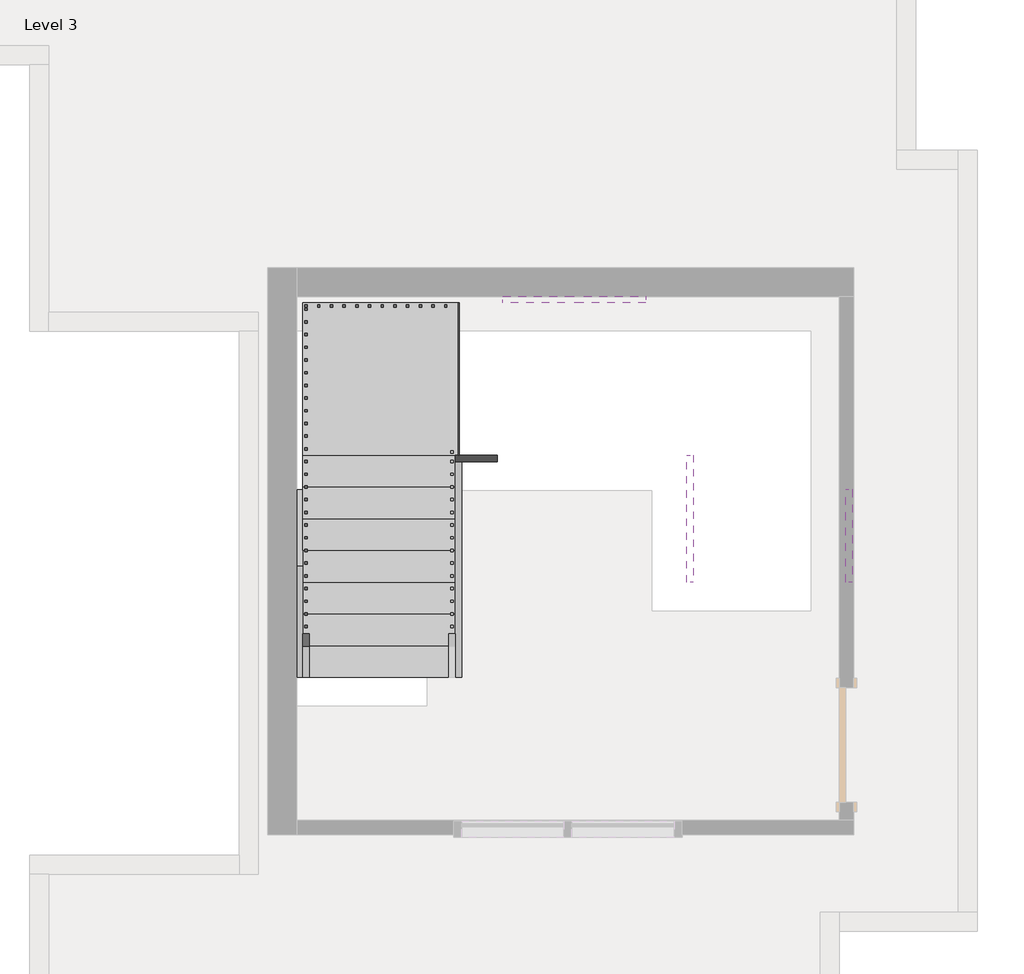
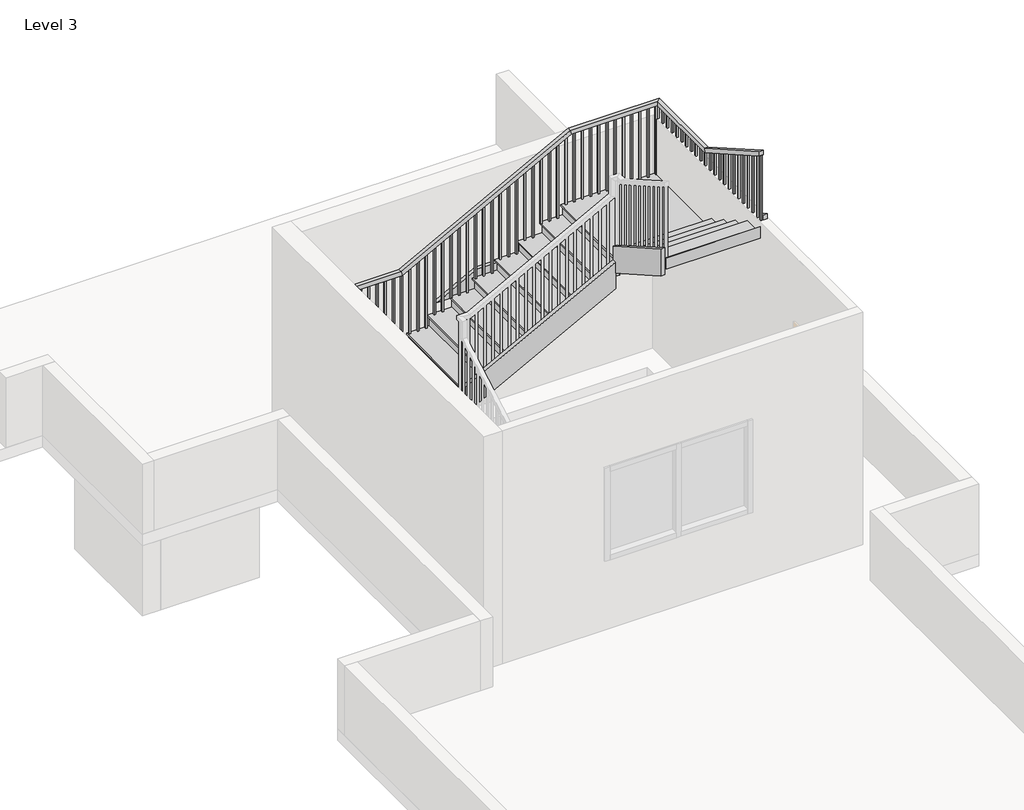
# One storey, part 2 of 2: 6 members, 1 railing, 1 stair flight.
"""IFC4 building model written with IfcOpenShell, lengths in millimetres."""

from ifc_helpers import new_model, si_unit, frame, origin, place, context, project, spatial, polyline, outline, extrude, faceted_brep, transform, mapped, element, save
from components import stair_flight_02d0fc9c

model = new_model("IFC4")

# Units and contexts
model_context = context("Model", 3, world=origin())
ifc_project = project(units=[si_unit("LENGTHUNIT", "METRE", prefix="MILLI")], contexts=[model_context])

# Site, building, storey
site = spatial("IfcSite", under=ifc_project)
building = spatial("IfcBuilding", under=site)
storey = spatial("IfcBuildingStorey", under=building, Name="Level 3", Elevation=6248.4)

# Members
placement = place(None, origin())
element("IfcMember", 1, ObjectType="Stringer - 2\" Width", at=placement, inside=storey, context=model_context, shape_type="SweptSolid", body=[
    extrude(outline(polyline([(12686.9618061, 6248.4), (12686.9618061, 6457.374685), (13575.3811074, 6965.0428571), (14189.7251478, 6965.0428571), (12935.6001478, 6248.4), (12686.9618061, 6248.4)])), frame((-40773.1146233, 0.0, 0.0), z_axis=(1.0, 0.0, 0.0), x_axis=(0.0, 1.0, 0.0)), (0.0, 0.0, 1.0), 50.8),
])
element("IfcMember", 2, ObjectType="Stringer - 2\" Width", at=placement, inside=storey, context=model_context, shape_type="SweptSolid", body=[
    extrude(outline(polyline([(7819.0066619, -38473.4324895), (8082.974685, -37978.4924462), (8082.974685, -38626.1924462), (7819.0066619, -39121.1324895), (7819.0066619, -38473.4324895)])), frame((0.0, 15684.1618061, 0.0), z_axis=(0.0, 1.0, 0.0), x_axis=(0.0, 0.0, 1.0)), (0.0, 0.0, 1.0), 50.8),
])
element("IfcMember", 3, ObjectType="Stringer - 2\" Width", at=placement, inside=storey, context=model_context, shape_type="SweptSolid", body=[
    extrude(outline(polyline([(13576.8784643, 8936.0828571), (13448.9618061, 9009.1780904), (13448.9618061, 9360.2318278), (14191.2225047, 8936.0828571), (13576.8784643, 8936.0828571)])), frame((-36378.9146233, 0.0, 0.0), z_axis=(1.0, 0.0, 0.0), x_axis=(0.0, 1.0, 0.0)), (0.0, 0.0, 1.0), 50.8),
])
element("IfcMember", 4, ObjectType="Stringer - 2\" Width", at=placement, inside=storey, context=model_context, shape_type="SweptSolid", body=[
    extrude(outline(polyline([(12686.9618061, 6248.4), (12686.9618061, 6457.374685), (14414.1618061, 7444.3461135), (14414.1618061, 7093.2923761), (12935.6001478, 6248.4), (12686.9618061, 6248.4)])), frame((-39503.1146233, 0.0, 0.0), z_axis=(1.0, 0.0, 0.0), x_axis=(0.0, 1.0, 0.0)), (0.0, 0.0, 1.0), 50.8),
])
element("IfcMember", 5, ObjectType="Stringer - 2\" Width", at=placement, inside=storey, context=model_context, shape_type="SweptSolid", body=[
    extrude(outline(polyline([(7615.2828571, -39503.1146233), (7269.8428571, -39503.1146233), (8258.7495238, -37648.9146233), (8604.1895238, -37648.9146233), (7615.2828571, -39503.1146233)])), frame((0.0, 14414.1618061, 0.0), z_axis=(0.0, 1.0, 0.0), x_axis=(0.0, 0.0, 1.0)), (0.0, 0.0, 1.0), 50.8),
])
element("IfcMember", 6, ObjectType="Stringer - 2\" Width", at=placement, inside=storey, context=model_context, shape_type="SweptSolid", body=[
    extrude(outline(polyline([(14464.9618061, 8779.6603992), (14464.9618061, 8428.6066619), (13448.9618061, 9009.1780904), (13448.9618061, 9360.2318278), (14464.9618061, 8779.6603992)])), frame((-37648.9146233, 0.0, 0.0), z_axis=(1.0, 0.0, 0.0), x_axis=(0.0, 1.0, 0.0)), (0.0, 0.0, 1.0), 50.8),
])

# Railing
element("IfcRailing", 7, ObjectType="Handrail - Rectangular", at=placement, inside=storey, context=model_context, shape_type="SolidModel", body=[
    faceted_brep([(-40722.3146233, 12686.9618061, 7307.9428571), (-40722.3146233, 12686.9618061, 7249.4339009), (-40671.5146233, 12686.9618061, 7249.4339009), (-40671.5146233, 12686.9618061, 7307.9428571), (-40722.3146233, 14631.7551394, 8419.2533333), (-40722.3146233, 14645.2458128, 8368.4533333), (-40671.5146233, 14645.2458128, 8368.4533333), (-40671.5146233, 14631.7551394, 8419.2533333), (-40722.3146233, 15684.1618061, 8419.2533333), (-40722.3146233, 15684.1618061, 8368.4533333), (-40671.5146233, 15633.3618061, 8368.4533333), (-40671.5146233, 15633.3618061, 8419.2533333), (-39596.5503376, 15684.1618061, 8419.2533333), (-39583.8503376, 15684.1618061, 8368.4533333), (-39583.8503376, 15633.3618061, 8368.4533333), (-39596.5503376, 15633.3618061, 8419.2533333), (-37504.6789091, 15684.1618061, 9534.9180952), (-37491.9789091, 15684.1618061, 9484.1180952), (-37491.9789091, 15633.3618061, 9484.1180952), (-37504.6789091, 15633.3618061, 9534.9180952), (-36378.9146233, 15684.1618061, 9534.9180952), (-36378.9146233, 15684.1618061, 9484.1180952), (-36429.7146233, 15633.3618061, 9484.1180952), (-36429.7146233, 15633.3618061, 9534.9180952), (-36378.9146233, 14631.7551394, 9534.9180952), (-36378.9146233, 14618.264466, 9484.1180952), (-36429.7146233, 14618.264466, 9484.1180952), (-36429.7146233, 14631.7551394, 9534.9180952), (-36378.9146233, 13448.9618061, 10210.8), (-36429.7146233, 13448.9618061, 10210.8), (-36429.7146233, 13448.9618061, 10152.2910438), (-36378.9146233, 13448.9618061, 10152.2910438)], [[[0, 1, 2, 3]], [[1, 0, 4, 5]], [[2, 1, 5, 6]], [[3, 2, 6, 7]], [[0, 3, 7, 4]], [[5, 4, 8, 9]], [[6, 5, 9, 10]], [[7, 6, 10, 11]], [[4, 7, 11, 8]], [[9, 8, 12, 13]], [[10, 9, 13, 14]], [[11, 10, 14, 15]], [[8, 11, 15, 12]], [[13, 12, 16, 17]], [[14, 13, 17, 18]], [[15, 14, 18, 19]], [[12, 15, 19, 16]], [[17, 16, 20, 21]], [[18, 17, 21, 22]], [[19, 18, 22, 23]], [[16, 19, 23, 20]], [[21, 20, 24, 25]], [[22, 21, 25, 26]], [[23, 22, 26, 27]], [[20, 23, 27, 24]], [[28, 29, 30, 31]], [[25, 24, 28, 31]], [[26, 25, 31, 30]], [[27, 26, 30, 29]], [[24, 27, 29, 28]]]),
    extrude(outline(polyline([(13534.6868061, 10103.3053295), (13534.6868061, 9151.2571429), (13515.6368061, 9151.2571429), (13515.6368061, 10114.1910438), (13534.6868061, 10103.3053295)])), frame((-36413.8396233, 0.0, 0.0), z_axis=(1.0, 0.0, 0.0), x_axis=(0.0, 1.0, 0.0)), (0.0, 0.0, 1.0), 19.05),
    extrude(outline(polyline([(13636.2868061, 10045.2481866), (13636.2868061, 9151.2571429), (13617.2368061, 9151.2571429), (13617.2368061, 10056.1339009), (13636.2868061, 10045.2481866)])), frame((-36413.8396233, 0.0, 0.0), z_axis=(1.0, 0.0, 0.0), x_axis=(0.0, 1.0, 0.0)), (0.0, 0.0, 1.0), 19.05),
    extrude(outline(polyline([(13737.8868061, 9987.1910438), (13737.8868061, 9006.1142857), (13718.8368061, 9006.1142857), (13718.8368061, 9998.0767581), (13737.8868061, 9987.1910438)])), frame((-36413.8396233, 0.0, 0.0), z_axis=(1.0, 0.0, 0.0), x_axis=(0.0, 1.0, 0.0)), (0.0, 0.0, 1.0), 19.05),
    extrude(outline(polyline([(13839.4868061, 9929.1339009), (13839.4868061, 9006.1142857), (13820.4368061, 9006.1142857), (13820.4368061, 9940.0196152), (13839.4868061, 9929.1339009)])), frame((-36413.8396233, 0.0, 0.0), z_axis=(1.0, 0.0, 0.0), x_axis=(0.0, 1.0, 0.0)), (0.0, 0.0, 1.0), 19.05),
    extrude(outline(polyline([(13941.0868061, 9871.0767581), (13941.0868061, 9006.1142857), (13922.0368061, 9006.1142857), (13922.0368061, 9881.9624723), (13941.0868061, 9871.0767581)])), frame((-36413.8396233, 0.0, 0.0), z_axis=(1.0, 0.0, 0.0), x_axis=(0.0, 1.0, 0.0)), (0.0, 0.0, 1.0), 19.05),
    extrude(outline(polyline([(14042.6868061, 9813.0196152), (14042.6868061, 8860.9714286), (14023.6368061, 8860.9714286), (14023.6368061, 9823.9053295), (14042.6868061, 9813.0196152)])), frame((-36413.8396233, 0.0, 0.0), z_axis=(1.0, 0.0, 0.0), x_axis=(0.0, 1.0, 0.0)), (0.0, 0.0, 1.0), 19.05),
    extrude(outline(polyline([(14144.2868061, 9754.9624723), (14144.2868061, 8860.9714286), (14125.2368061, 8860.9714286), (14125.2368061, 9765.8481866), (14144.2868061, 9754.9624723)])), frame((-36413.8396233, 0.0, 0.0), z_axis=(1.0, 0.0, 0.0), x_axis=(0.0, 1.0, 0.0)), (0.0, 0.0, 1.0), 19.05),
    extrude(outline(polyline([(14245.8868061, 9696.9053295), (14245.8868061, 8715.8285714), (14226.8368061, 8715.8285714), (14226.8368061, 9707.7910438), (14245.8868061, 9696.9053295)])), frame((-36413.8396233, 0.0, 0.0), z_axis=(1.0, 0.0, 0.0), x_axis=(0.0, 1.0, 0.0)), (0.0, 0.0, 1.0), 19.05),
    extrude(outline(polyline([(14347.4868061, 9638.8481866), (14347.4868061, 8715.8285714), (14328.4368061, 8715.8285714), (14328.4368061, 9649.7339009), (14347.4868061, 9638.8481866)])), frame((-36413.8396233, 0.0, 0.0), z_axis=(1.0, 0.0, 0.0), x_axis=(0.0, 1.0, 0.0)), (0.0, 0.0, 1.0), 19.05),
    extrude(outline(polyline([(14449.0868061, 9580.7910438), (14449.0868061, 8715.8285714), (14430.0368061, 8715.8285714), (14430.0368061, 9591.6767581), (14449.0868061, 9580.7910438)])), frame((-36413.8396233, 0.0, 0.0), z_axis=(1.0, 0.0, 0.0), x_axis=(0.0, 1.0, 0.0)), (0.0, 0.0, 1.0), 19.05),
    extrude(outline(polyline([(14550.6868061, 9522.7339009), (14550.6868061, 8570.6857143), (14531.6368061, 8570.6857143), (14531.6368061, 9533.6196152), (14550.6868061, 9522.7339009)])), frame((-36413.8396233, 0.0, 0.0), z_axis=(1.0, 0.0, 0.0), x_axis=(0.0, 1.0, 0.0)), (0.0, 0.0, 1.0), 19.05),
    extrude(outline(polyline([(-36394.7896233, 14652.2868061), (-36394.7896233, 14633.2368061), (-36413.8396233, 14633.2368061), (-36413.8396233, 14652.2868061), (-36394.7896233, 14652.2868061)])), frame((0.0, 0.0, 8570.6857143), z_axis=(0.0, 0.0, 1.0), x_axis=(1.0, 0.0, 0.0)), (0.0, 0.0, 1.0), 913.432381),
    extrude(outline(polyline([(-36394.7896233, 14753.8868061), (-36394.7896233, 14734.8368061), (-36413.8396233, 14734.8368061), (-36413.8396233, 14753.8868061), (-36394.7896233, 14753.8868061)])), frame((0.0, 0.0, 8570.6857143), z_axis=(0.0, 0.0, 1.0), x_axis=(1.0, 0.0, 0.0)), (0.0, 0.0, 1.0), 913.432381),
    extrude(outline(polyline([(-36394.7896233, 14855.4868061), (-36394.7896233, 14836.4368061), (-36413.8396233, 14836.4368061), (-36413.8396233, 14855.4868061), (-36394.7896233, 14855.4868061)])), frame((0.0, 0.0, 8570.6857143), z_axis=(0.0, 0.0, 1.0), x_axis=(1.0, 0.0, 0.0)), (0.0, 0.0, 1.0), 913.432381),
    extrude(outline(polyline([(-36394.7896233, 14957.0868061), (-36394.7896233, 14938.0368061), (-36413.8396233, 14938.0368061), (-36413.8396233, 14957.0868061), (-36394.7896233, 14957.0868061)])), frame((0.0, 0.0, 8570.6857143), z_axis=(0.0, 0.0, 1.0), x_axis=(1.0, 0.0, 0.0)), (0.0, 0.0, 1.0), 913.432381),
    extrude(outline(polyline([(-36394.7896233, 15058.6868061), (-36394.7896233, 15039.6368061), (-36413.8396233, 15039.6368061), (-36413.8396233, 15058.6868061), (-36394.7896233, 15058.6868061)])), frame((0.0, 0.0, 8570.6857143), z_axis=(0.0, 0.0, 1.0), x_axis=(1.0, 0.0, 0.0)), (0.0, 0.0, 1.0), 913.432381),
    extrude(outline(polyline([(-36394.7896233, 15160.2868061), (-36394.7896233, 15141.2368061), (-36413.8396233, 15141.2368061), (-36413.8396233, 15160.2868061), (-36394.7896233, 15160.2868061)])), frame((0.0, 0.0, 8570.6857143), z_axis=(0.0, 0.0, 1.0), x_axis=(1.0, 0.0, 0.0)), (0.0, 0.0, 1.0), 913.432381),
    extrude(outline(polyline([(-36394.7896233, 15261.8868061), (-36394.7896233, 15242.8368061), (-36413.8396233, 15242.8368061), (-36413.8396233, 15261.8868061), (-36394.7896233, 15261.8868061)])), frame((0.0, 0.0, 8570.6857143), z_axis=(0.0, 0.0, 1.0), x_axis=(1.0, 0.0, 0.0)), (0.0, 0.0, 1.0), 913.432381),
    extrude(outline(polyline([(-36394.7896233, 15363.4868061), (-36394.7896233, 15344.4368061), (-36413.8396233, 15344.4368061), (-36413.8396233, 15363.4868061), (-36394.7896233, 15363.4868061)])), frame((0.0, 0.0, 8570.6857143), z_axis=(0.0, 0.0, 1.0), x_axis=(1.0, 0.0, 0.0)), (0.0, 0.0, 1.0), 913.432381),
    extrude(outline(polyline([(-36394.7896233, 15465.0868061), (-36394.7896233, 15446.0368061), (-36413.8396233, 15446.0368061), (-36413.8396233, 15465.0868061), (-36394.7896233, 15465.0868061)])), frame((0.0, 0.0, 8570.6857143), z_axis=(0.0, 0.0, 1.0), x_axis=(1.0, 0.0, 0.0)), (0.0, 0.0, 1.0), 913.432381),
    extrude(outline(polyline([(-36394.7896233, 15566.6868061), (-36394.7896233, 15547.6368061), (-36413.8396233, 15547.6368061), (-36413.8396233, 15566.6868061), (-36394.7896233, 15566.6868061)])), frame((0.0, 0.0, 8570.6857143), z_axis=(0.0, 0.0, 1.0), x_axis=(1.0, 0.0, 0.0)), (0.0, 0.0, 1.0), 913.432381),
    extrude(outline(polyline([(-36439.2396233, 15668.2868061), (-36420.1896233, 15668.2868061), (-36420.1896233, 15649.2368061), (-36439.2396233, 15649.2368061), (-36439.2396233, 15668.2868061)])), frame((0.0, 0.0, 8570.6857143), z_axis=(0.0, 0.0, 1.0), x_axis=(1.0, 0.0, 0.0)), (0.0, 0.0, 1.0), 913.432381),
    extrude(outline(polyline([(-36540.8396233, 15668.2868061), (-36521.7896233, 15668.2868061), (-36521.7896233, 15649.2368061), (-36540.8396233, 15649.2368061), (-36540.8396233, 15668.2868061)])), frame((0.0, 0.0, 8570.6857143), z_axis=(0.0, 0.0, 1.0), x_axis=(1.0, 0.0, 0.0)), (0.0, 0.0, 1.0), 913.432381),
    extrude(outline(polyline([(-36642.4396233, 15668.2868061), (-36623.3896233, 15668.2868061), (-36623.3896233, 15649.2368061), (-36642.4396233, 15649.2368061), (-36642.4396233, 15668.2868061)])), frame((0.0, 0.0, 8570.6857143), z_axis=(0.0, 0.0, 1.0), x_axis=(1.0, 0.0, 0.0)), (0.0, 0.0, 1.0), 913.432381),
    extrude(outline(polyline([(-36744.0396233, 15668.2868061), (-36724.9896233, 15668.2868061), (-36724.9896233, 15649.2368061), (-36744.0396233, 15649.2368061), (-36744.0396233, 15668.2868061)])), frame((0.0, 0.0, 8570.6857143), z_axis=(0.0, 0.0, 1.0), x_axis=(1.0, 0.0, 0.0)), (0.0, 0.0, 1.0), 913.432381),
    extrude(outline(polyline([(-36845.6396233, 15668.2868061), (-36826.5896233, 15668.2868061), (-36826.5896233, 15649.2368061), (-36845.6396233, 15649.2368061), (-36845.6396233, 15668.2868061)])), frame((0.0, 0.0, 8570.6857143), z_axis=(0.0, 0.0, 1.0), x_axis=(1.0, 0.0, 0.0)), (0.0, 0.0, 1.0), 913.432381),
    extrude(outline(polyline([(-36947.2396233, 15668.2868061), (-36928.1896233, 15668.2868061), (-36928.1896233, 15649.2368061), (-36947.2396233, 15649.2368061), (-36947.2396233, 15668.2868061)])), frame((0.0, 0.0, 8570.6857143), z_axis=(0.0, 0.0, 1.0), x_axis=(1.0, 0.0, 0.0)), (0.0, 0.0, 1.0), 913.432381),
    extrude(outline(polyline([(-37048.8396233, 15668.2868061), (-37029.7896233, 15668.2868061), (-37029.7896233, 15649.2368061), (-37048.8396233, 15649.2368061), (-37048.8396233, 15668.2868061)])), frame((0.0, 0.0, 8570.6857143), z_axis=(0.0, 0.0, 1.0), x_axis=(1.0, 0.0, 0.0)), (0.0, 0.0, 1.0), 913.432381),
    extrude(outline(polyline([(-37150.4396233, 15668.2868061), (-37131.3896233, 15668.2868061), (-37131.3896233, 15649.2368061), (-37150.4396233, 15649.2368061), (-37150.4396233, 15668.2868061)])), frame((0.0, 0.0, 8570.6857143), z_axis=(0.0, 0.0, 1.0), x_axis=(1.0, 0.0, 0.0)), (0.0, 0.0, 1.0), 913.432381),
    extrude(outline(polyline([(-37252.0396233, 15668.2868061), (-37232.9896233, 15668.2868061), (-37232.9896233, 15649.2368061), (-37252.0396233, 15649.2368061), (-37252.0396233, 15668.2868061)])), frame((0.0, 0.0, 8570.6857143), z_axis=(0.0, 0.0, 1.0), x_axis=(1.0, 0.0, 0.0)), (0.0, 0.0, 1.0), 913.432381),
    extrude(outline(polyline([(-37353.6396233, 15668.2868061), (-37334.5896233, 15668.2868061), (-37334.5896233, 15649.2368061), (-37353.6396233, 15649.2368061), (-37353.6396233, 15668.2868061)])), frame((0.0, 0.0, 8570.6857143), z_axis=(0.0, 0.0, 1.0), x_axis=(1.0, 0.0, 0.0)), (0.0, 0.0, 1.0), 913.432381),
    extrude(outline(polyline([(-37455.2396233, 15668.2868061), (-37436.1896233, 15668.2868061), (-37436.1896233, 15649.2368061), (-37455.2396233, 15649.2368061), (-37455.2396233, 15668.2868061)])), frame((0.0, 0.0, 8570.6857143), z_axis=(0.0, 0.0, 1.0), x_axis=(1.0, 0.0, 0.0)), (0.0, 0.0, 1.0), 913.432381),
    extrude(outline(polyline([(9449.5257143, -37556.8396233), (8570.6857143, -37556.8396233), (8570.6857143, -37537.7896233), (9459.6857143, -37537.7896233), (9449.5257143, -37556.8396233)])), frame((0.0, 15649.2368061, 0.0), z_axis=(0.0, 1.0, 0.0), x_axis=(0.0, 0.0, 1.0)), (0.0, 0.0, 1.0), 19.05),
    extrude(outline(polyline([(9395.3390476, -37658.4396233), (8425.5428571, -37658.4396233), (8425.5428571, -37639.3896233), (9405.4990476, -37639.3896233), (9395.3390476, -37658.4396233)])), frame((0.0, 15649.2368061, 0.0), z_axis=(0.0, 1.0, 0.0), x_axis=(0.0, 0.0, 1.0)), (0.0, 0.0, 1.0), 19.05),
    extrude(outline(polyline([(9341.152381, -37760.0396233), (8425.5428571, -37760.0396233), (8425.5428571, -37740.9896233), (9351.312381, -37740.9896233), (9341.152381, -37760.0396233)])), frame((0.0, 15649.2368061, 0.0), z_axis=(0.0, 1.0, 0.0), x_axis=(0.0, 0.0, 1.0)), (0.0, 0.0, 1.0), 19.05),
    extrude(outline(polyline([(9286.9657143, -37861.6396233), (8425.5428571, -37861.6396233), (8425.5428571, -37842.5896233), (9297.1257143, -37842.5896233), (9286.9657143, -37861.6396233)])), frame((0.0, 15649.2368061, 0.0), z_axis=(0.0, 1.0, 0.0), x_axis=(0.0, 0.0, 1.0)), (0.0, 0.0, 1.0), 19.05),
    extrude(outline(polyline([(9232.7790476, -37963.2396233), (8280.4, -37963.2396233), (8280.4, -37944.1896233), (9242.9390476, -37944.1896233), (9232.7790476, -37963.2396233)])), frame((0.0, 15649.2368061, 0.0), z_axis=(0.0, 1.0, 0.0), x_axis=(0.0, 0.0, 1.0)), (0.0, 0.0, 1.0), 19.05),
    extrude(outline(polyline([(9178.592381, -38064.8396233), (8280.4, -38064.8396233), (8280.4, -38045.7896233), (9188.752381, -38045.7896233), (9178.592381, -38064.8396233)])), frame((0.0, 15649.2368061, 0.0), z_axis=(0.0, 1.0, 0.0), x_axis=(0.0, 0.0, 1.0)), (0.0, 0.0, 1.0), 19.05),
    extrude(outline(polyline([(9124.4057143, -38166.4396233), (8135.2571429, -38166.4396233), (8135.2571429, -38147.3896233), (9134.5657143, -38147.3896233), (9124.4057143, -38166.4396233)])), frame((0.0, 15649.2368061, 0.0), z_axis=(0.0, 1.0, 0.0), x_axis=(0.0, 0.0, 1.0)), (0.0, 0.0, 1.0), 19.05),
    extrude(outline(polyline([(9070.2190476, -38268.0396233), (8135.2571429, -38268.0396233), (8135.2571429, -38248.9896233), (9080.3790476, -38248.9896233), (9070.2190476, -38268.0396233)])), frame((0.0, 15649.2368061, 0.0), z_axis=(0.0, 1.0, 0.0), x_axis=(0.0, 0.0, 1.0)), (0.0, 0.0, 1.0), 19.05),
    extrude(outline(polyline([(9016.032381, -38369.6396233), (8135.2571429, -38369.6396233), (8135.2571429, -38350.5896233), (9026.192381, -38350.5896233), (9016.032381, -38369.6396233)])), frame((0.0, 15649.2368061, 0.0), z_axis=(0.0, 1.0, 0.0), x_axis=(0.0, 0.0, 1.0)), (0.0, 0.0, 1.0), 19.05),
    extrude(outline(polyline([(8961.8457143, -38471.2396233), (7990.1142857, -38471.2396233), (7990.1142857, -38452.1896233), (8972.0057143, -38452.1896233), (8961.8457143, -38471.2396233)])), frame((0.0, 15649.2368061, 0.0), z_axis=(0.0, 1.0, 0.0), x_axis=(0.0, 0.0, 1.0)), (0.0, 0.0, 1.0), 19.05),
    extrude(outline(polyline([(8907.6590476, -38572.8396233), (7990.1142857, -38572.8396233), (7990.1142857, -38553.7896233), (8917.8190476, -38553.7896233), (8907.6590476, -38572.8396233)])), frame((0.0, 15649.2368061, 0.0), z_axis=(0.0, 1.0, 0.0), x_axis=(0.0, 0.0, 1.0)), (0.0, 0.0, 1.0), 19.05),
    extrude(outline(polyline([(8853.472381, -38674.4396233), (7990.1142857, -38674.4396233), (7990.1142857, -38655.3896233), (8863.632381, -38655.3896233), (8853.472381, -38674.4396233)])), frame((0.0, 15649.2368061, 0.0), z_axis=(0.0, 1.0, 0.0), x_axis=(0.0, 0.0, 1.0)), (0.0, 0.0, 1.0), 19.05),
    extrude(outline(polyline([(8799.2857143, -38776.0396233), (7844.9714286, -38776.0396233), (7844.9714286, -38756.9896233), (8809.4457143, -38756.9896233), (8799.2857143, -38776.0396233)])), frame((0.0, 15649.2368061, 0.0), z_axis=(0.0, 1.0, 0.0), x_axis=(0.0, 0.0, 1.0)), (0.0, 0.0, 1.0), 19.05),
    extrude(outline(polyline([(8745.0990476, -38877.6396233), (7844.9714286, -38877.6396233), (7844.9714286, -38858.5896233), (8755.2590476, -38858.5896233), (8745.0990476, -38877.6396233)])), frame((0.0, 15649.2368061, 0.0), z_axis=(0.0, 1.0, 0.0), x_axis=(0.0, 0.0, 1.0)), (0.0, 0.0, 1.0), 19.05),
    extrude(outline(polyline([(8690.912381, -38979.2396233), (7844.9714286, -38979.2396233), (7844.9714286, -38960.1896233), (8701.072381, -38960.1896233), (8690.912381, -38979.2396233)])), frame((0.0, 15649.2368061, 0.0), z_axis=(0.0, 1.0, 0.0), x_axis=(0.0, 0.0, 1.0)), (0.0, 0.0, 1.0), 19.05),
    extrude(outline(polyline([(8636.7257143, -39080.8396233), (7699.8285714, -39080.8396233), (7699.8285714, -39061.7896233), (8646.8857143, -39061.7896233), (8636.7257143, -39080.8396233)])), frame((0.0, 15649.2368061, 0.0), z_axis=(0.0, 1.0, 0.0), x_axis=(0.0, 0.0, 1.0)), (0.0, 0.0, 1.0), 19.05),
    extrude(outline(polyline([(8582.5390476, -39182.4396233), (7699.8285714, -39182.4396233), (7699.8285714, -39163.3896233), (8592.6990476, -39163.3896233), (8582.5390476, -39182.4396233)])), frame((0.0, 15649.2368061, 0.0), z_axis=(0.0, 1.0, 0.0), x_axis=(0.0, 0.0, 1.0)), (0.0, 0.0, 1.0), 19.05),
    extrude(outline(polyline([(8528.352381, -39284.0396233), (7554.6857143, -39284.0396233), (7554.6857143, -39264.9896233), (8538.512381, -39264.9896233), (8528.352381, -39284.0396233)])), frame((0.0, 15649.2368061, 0.0), z_axis=(0.0, 1.0, 0.0), x_axis=(0.0, 0.0, 1.0)), (0.0, 0.0, 1.0), 19.05),
    extrude(outline(polyline([(8474.1657143, -39385.6396233), (7554.6857143, -39385.6396233), (7554.6857143, -39366.5896233), (8484.3257143, -39366.5896233), (8474.1657143, -39385.6396233)])), frame((0.0, 15649.2368061, 0.0), z_axis=(0.0, 1.0, 0.0), x_axis=(0.0, 0.0, 1.0)), (0.0, 0.0, 1.0), 19.05),
    extrude(outline(polyline([(8419.9790476, -39487.2396233), (7554.6857143, -39487.2396233), (7554.6857143, -39468.1896233), (8430.1390476, -39468.1896233), (8419.9790476, -39487.2396233)])), frame((0.0, 15649.2368061, 0.0), z_axis=(0.0, 1.0, 0.0), x_axis=(0.0, 0.0, 1.0)), (0.0, 0.0, 1.0), 19.05),
    extrude(outline(polyline([(8365.792381, -39588.8396233), (7409.5428571, -39588.8396233), (7409.5428571, -39569.7896233), (8375.952381, -39569.7896233), (8365.792381, -39588.8396233)])), frame((0.0, 15649.2368061, 0.0), z_axis=(0.0, 1.0, 0.0), x_axis=(0.0, 0.0, 1.0)), (0.0, 0.0, 1.0), 19.05),
    extrude(outline(polyline([(-39690.4396233, 15668.2868061), (-39671.3896233, 15668.2868061), (-39671.3896233, 15649.2368061), (-39690.4396233, 15649.2368061), (-39690.4396233, 15668.2868061)])), frame((0.0, 0.0, 7409.5428571), z_axis=(0.0, 0.0, 1.0), x_axis=(1.0, 0.0, 0.0)), (0.0, 0.0, 1.0), 958.9104762),
    extrude(outline(polyline([(-39792.0396233, 15668.2868061), (-39772.9896233, 15668.2868061), (-39772.9896233, 15649.2368061), (-39792.0396233, 15649.2368061), (-39792.0396233, 15668.2868061)])), frame((0.0, 0.0, 7409.5428571), z_axis=(0.0, 0.0, 1.0), x_axis=(1.0, 0.0, 0.0)), (0.0, 0.0, 1.0), 958.9104762),
    extrude(outline(polyline([(-39893.6396233, 15668.2868061), (-39874.5896233, 15668.2868061), (-39874.5896233, 15649.2368061), (-39893.6396233, 15649.2368061), (-39893.6396233, 15668.2868061)])), frame((0.0, 0.0, 7409.5428571), z_axis=(0.0, 0.0, 1.0), x_axis=(1.0, 0.0, 0.0)), (0.0, 0.0, 1.0), 958.9104762),
    extrude(outline(polyline([(-39995.2396233, 15668.2868061), (-39976.1896233, 15668.2868061), (-39976.1896233, 15649.2368061), (-39995.2396233, 15649.2368061), (-39995.2396233, 15668.2868061)])), frame((0.0, 0.0, 7409.5428571), z_axis=(0.0, 0.0, 1.0), x_axis=(1.0, 0.0, 0.0)), (0.0, 0.0, 1.0), 958.9104762),
    extrude(outline(polyline([(-40096.8396233, 15668.2868061), (-40077.7896233, 15668.2868061), (-40077.7896233, 15649.2368061), (-40096.8396233, 15649.2368061), (-40096.8396233, 15668.2868061)])), frame((0.0, 0.0, 7409.5428571), z_axis=(0.0, 0.0, 1.0), x_axis=(1.0, 0.0, 0.0)), (0.0, 0.0, 1.0), 958.9104762),
    extrude(outline(polyline([(-40198.4396233, 15668.2868061), (-40179.3896233, 15668.2868061), (-40179.3896233, 15649.2368061), (-40198.4396233, 15649.2368061), (-40198.4396233, 15668.2868061)])), frame((0.0, 0.0, 7409.5428571), z_axis=(0.0, 0.0, 1.0), x_axis=(1.0, 0.0, 0.0)), (0.0, 0.0, 1.0), 958.9104762),
    extrude(outline(polyline([(-40300.0396233, 15668.2868061), (-40280.9896233, 15668.2868061), (-40280.9896233, 15649.2368061), (-40300.0396233, 15649.2368061), (-40300.0396233, 15668.2868061)])), frame((0.0, 0.0, 7409.5428571), z_axis=(0.0, 0.0, 1.0), x_axis=(1.0, 0.0, 0.0)), (0.0, 0.0, 1.0), 958.9104762),
    extrude(outline(polyline([(-40401.6396233, 15668.2868061), (-40382.5896233, 15668.2868061), (-40382.5896233, 15649.2368061), (-40401.6396233, 15649.2368061), (-40401.6396233, 15668.2868061)])), frame((0.0, 0.0, 7409.5428571), z_axis=(0.0, 0.0, 1.0), x_axis=(1.0, 0.0, 0.0)), (0.0, 0.0, 1.0), 958.9104762),
    extrude(outline(polyline([(-40503.2396233, 15668.2868061), (-40484.1896233, 15668.2868061), (-40484.1896233, 15649.2368061), (-40503.2396233, 15649.2368061), (-40503.2396233, 15668.2868061)])), frame((0.0, 0.0, 7409.5428571), z_axis=(0.0, 0.0, 1.0), x_axis=(1.0, 0.0, 0.0)), (0.0, 0.0, 1.0), 958.9104762),
    extrude(outline(polyline([(-40604.8396233, 15668.2868061), (-40585.7896233, 15668.2868061), (-40585.7896233, 15649.2368061), (-40604.8396233, 15649.2368061), (-40604.8396233, 15668.2868061)])), frame((0.0, 0.0, 7409.5428571), z_axis=(0.0, 0.0, 1.0), x_axis=(1.0, 0.0, 0.0)), (0.0, 0.0, 1.0), 958.9104762),
    extrude(outline(polyline([(-40706.4396233, 15623.8368061), (-40706.4396233, 15642.8868061), (-40687.3896233, 15642.8868061), (-40687.3896233, 15623.8368061), (-40706.4396233, 15623.8368061)])), frame((0.0, 0.0, 7409.5428571), z_axis=(0.0, 0.0, 1.0), x_axis=(1.0, 0.0, 0.0)), (0.0, 0.0, 1.0), 958.9104762),
    extrude(outline(polyline([(-40706.4396233, 15522.2368061), (-40706.4396233, 15541.2868061), (-40687.3896233, 15541.2868061), (-40687.3896233, 15522.2368061), (-40706.4396233, 15522.2368061)])), frame((0.0, 0.0, 7409.5428571), z_axis=(0.0, 0.0, 1.0), x_axis=(1.0, 0.0, 0.0)), (0.0, 0.0, 1.0), 958.9104762),
    extrude(outline(polyline([(-40706.4396233, 15420.6368061), (-40706.4396233, 15439.6868061), (-40687.3896233, 15439.6868061), (-40687.3896233, 15420.6368061), (-40706.4396233, 15420.6368061)])), frame((0.0, 0.0, 7409.5428571), z_axis=(0.0, 0.0, 1.0), x_axis=(1.0, 0.0, 0.0)), (0.0, 0.0, 1.0), 958.9104762),
    extrude(outline(polyline([(-40706.4396233, 15319.0368061), (-40706.4396233, 15338.0868061), (-40687.3896233, 15338.0868061), (-40687.3896233, 15319.0368061), (-40706.4396233, 15319.0368061)])), frame((0.0, 0.0, 7409.5428571), z_axis=(0.0, 0.0, 1.0), x_axis=(1.0, 0.0, 0.0)), (0.0, 0.0, 1.0), 958.9104762),
    extrude(outline(polyline([(-40706.4396233, 15217.4368061), (-40706.4396233, 15236.4868061), (-40687.3896233, 15236.4868061), (-40687.3896233, 15217.4368061), (-40706.4396233, 15217.4368061)])), frame((0.0, 0.0, 7409.5428571), z_axis=(0.0, 0.0, 1.0), x_axis=(1.0, 0.0, 0.0)), (0.0, 0.0, 1.0), 958.9104762),
    extrude(outline(polyline([(-40706.4396233, 15115.8368061), (-40706.4396233, 15134.8868061), (-40687.3896233, 15134.8868061), (-40687.3896233, 15115.8368061), (-40706.4396233, 15115.8368061)])), frame((0.0, 0.0, 7409.5428571), z_axis=(0.0, 0.0, 1.0), x_axis=(1.0, 0.0, 0.0)), (0.0, 0.0, 1.0), 958.9104762),
    extrude(outline(polyline([(-40706.4396233, 15014.2368061), (-40706.4396233, 15033.2868061), (-40687.3896233, 15033.2868061), (-40687.3896233, 15014.2368061), (-40706.4396233, 15014.2368061)])), frame((0.0, 0.0, 7409.5428571), z_axis=(0.0, 0.0, 1.0), x_axis=(1.0, 0.0, 0.0)), (0.0, 0.0, 1.0), 958.9104762),
    extrude(outline(polyline([(-40706.4396233, 14912.6368061), (-40706.4396233, 14931.6868061), (-40687.3896233, 14931.6868061), (-40687.3896233, 14912.6368061), (-40706.4396233, 14912.6368061)])), frame((0.0, 0.0, 7409.5428571), z_axis=(0.0, 0.0, 1.0), x_axis=(1.0, 0.0, 0.0)), (0.0, 0.0, 1.0), 958.9104762),
    extrude(outline(polyline([(-40706.4396233, 14811.0368061), (-40706.4396233, 14830.0868061), (-40687.3896233, 14830.0868061), (-40687.3896233, 14811.0368061), (-40706.4396233, 14811.0368061)])), frame((0.0, 0.0, 7409.5428571), z_axis=(0.0, 0.0, 1.0), x_axis=(1.0, 0.0, 0.0)), (0.0, 0.0, 1.0), 958.9104762),
    extrude(outline(polyline([(-40706.4396233, 14709.4368061), (-40706.4396233, 14728.4868061), (-40687.3896233, 14728.4868061), (-40687.3896233, 14709.4368061), (-40706.4396233, 14709.4368061)])), frame((0.0, 0.0, 7409.5428571), z_axis=(0.0, 0.0, 1.0), x_axis=(1.0, 0.0, 0.0)), (0.0, 0.0, 1.0), 958.9104762),
    extrude(outline(polyline([(14626.8868061, 8357.9624723), (14626.8868061, 7409.5428571), (14607.8368061, 7409.5428571), (14607.8368061, 8347.0767581), (14626.8868061, 8357.9624723)])), frame((-40706.4396233, 0.0, 0.0), z_axis=(1.0, 0.0, 0.0), x_axis=(0.0, 1.0, 0.0)), (0.0, 0.0, 1.0), 19.05),
    extrude(outline(polyline([(14525.2868061, 8299.9053295), (14525.2868061, 7409.5428571), (14506.2368061, 7409.5428571), (14506.2368061, 8289.0196152), (14525.2868061, 8299.9053295)])), frame((-40706.4396233, 0.0, 0.0), z_axis=(1.0, 0.0, 0.0), x_axis=(0.0, 1.0, 0.0)), (0.0, 0.0, 1.0), 19.05),
    extrude(outline(polyline([(14423.6868061, 8241.8481866), (14423.6868061, 7264.4), (14404.6368061, 7264.4), (14404.6368061, 8230.9624723), (14423.6868061, 8241.8481866)])), frame((-40706.4396233, 0.0, 0.0), z_axis=(1.0, 0.0, 0.0), x_axis=(0.0, 1.0, 0.0)), (0.0, 0.0, 1.0), 19.05),
    extrude(outline(polyline([(14322.0868061, 8183.7910438), (14322.0868061, 7264.4), (14303.0368061, 7264.4), (14303.0368061, 8172.9053295), (14322.0868061, 8183.7910438)])), frame((-40706.4396233, 0.0, 0.0), z_axis=(1.0, 0.0, 0.0), x_axis=(0.0, 1.0, 0.0)), (0.0, 0.0, 1.0), 19.05),
    extrude(outline(polyline([(14220.4868061, 8125.7339009), (14220.4868061, 7264.4), (14201.4368061, 7264.4), (14201.4368061, 8114.8481866), (14220.4868061, 8125.7339009)])), frame((-40706.4396233, 0.0, 0.0), z_axis=(1.0, 0.0, 0.0), x_axis=(0.0, 1.0, 0.0)), (0.0, 0.0, 1.0), 19.05),
    extrude(outline(polyline([(14118.8868061, 8067.6767581), (14118.8868061, 7119.2571429), (14099.8368061, 7119.2571429), (14099.8368061, 8056.7910438), (14118.8868061, 8067.6767581)])), frame((-40706.4396233, 0.0, 0.0), z_axis=(1.0, 0.0, 0.0), x_axis=(0.0, 1.0, 0.0)), (0.0, 0.0, 1.0), 19.05),
    extrude(outline(polyline([(14017.2868061, 8009.6196152), (14017.2868061, 7119.2571429), (13998.2368061, 7119.2571429), (13998.2368061, 7998.7339009), (14017.2868061, 8009.6196152)])), frame((-40706.4396233, 0.0, 0.0), z_axis=(1.0, 0.0, 0.0), x_axis=(0.0, 1.0, 0.0)), (0.0, 0.0, 1.0), 19.05),
    extrude(outline(polyline([(13915.6868061, 7951.5624723), (13915.6868061, 6974.1142857), (13896.6368061, 6974.1142857), (13896.6368061, 7940.6767581), (13915.6868061, 7951.5624723)])), frame((-40706.4396233, 0.0, 0.0), z_axis=(1.0, 0.0, 0.0), x_axis=(0.0, 1.0, 0.0)), (0.0, 0.0, 1.0), 19.05),
    extrude(outline(polyline([(13814.0868061, 7893.5053295), (13814.0868061, 6974.1142857), (13795.0368061, 6974.1142857), (13795.0368061, 7882.6196152), (13814.0868061, 7893.5053295)])), frame((-40706.4396233, 0.0, 0.0), z_axis=(1.0, 0.0, 0.0), x_axis=(0.0, 1.0, 0.0)), (0.0, 0.0, 1.0), 19.05),
    extrude(outline(polyline([(13712.4868061, 7835.4481866), (13712.4868061, 6974.1142857), (13693.4368061, 6974.1142857), (13693.4368061, 7824.5624723), (13712.4868061, 7835.4481866)])), frame((-40706.4396233, 0.0, 0.0), z_axis=(1.0, 0.0, 0.0), x_axis=(0.0, 1.0, 0.0)), (0.0, 0.0, 1.0), 19.05),
    extrude(outline(polyline([(13610.8868061, 7777.3910438), (13610.8868061, 6828.9714286), (13591.8368061, 6828.9714286), (13591.8368061, 7766.5053295), (13610.8868061, 7777.3910438)])), frame((-40706.4396233, 0.0, 0.0), z_axis=(1.0, 0.0, 0.0), x_axis=(0.0, 1.0, 0.0)), (0.0, 0.0, 1.0), 19.05),
    extrude(outline(polyline([(13509.2868061, 7719.3339009), (13509.2868061, 6828.9714286), (13490.2368061, 6828.9714286), (13490.2368061, 7708.4481866), (13509.2868061, 7719.3339009)])), frame((-40706.4396233, 0.0, 0.0), z_axis=(1.0, 0.0, 0.0), x_axis=(0.0, 1.0, 0.0)), (0.0, 0.0, 1.0), 19.05),
    extrude(outline(polyline([(13407.6868061, 7661.2767581), (13407.6868061, 6683.8285714), (13388.6368061, 6683.8285714), (13388.6368061, 7650.3910438), (13407.6868061, 7661.2767581)])), frame((-40706.4396233, 0.0, 0.0), z_axis=(1.0, 0.0, 0.0), x_axis=(0.0, 1.0, 0.0)), (0.0, 0.0, 1.0), 19.05),
    extrude(outline(polyline([(13306.0868061, 7603.2196152), (13306.0868061, 6683.8285714), (13287.0368061, 6683.8285714), (13287.0368061, 7592.3339009), (13306.0868061, 7603.2196152)])), frame((-40706.4396233, 0.0, 0.0), z_axis=(1.0, 0.0, 0.0), x_axis=(0.0, 1.0, 0.0)), (0.0, 0.0, 1.0), 19.05),
    extrude(outline(polyline([(13204.4868061, 7545.1624723), (13204.4868061, 6683.8285714), (13185.4368061, 6683.8285714), (13185.4368061, 7534.2767581), (13204.4868061, 7545.1624723)])), frame((-40706.4396233, 0.0, 0.0), z_axis=(1.0, 0.0, 0.0), x_axis=(0.0, 1.0, 0.0)), (0.0, 0.0, 1.0), 19.05),
    extrude(outline(polyline([(13102.8868061, 7487.1053295), (13102.8868061, 6538.6857143), (13083.8368061, 6538.6857143), (13083.8368061, 7476.2196152), (13102.8868061, 7487.1053295)])), frame((-40706.4396233, 0.0, 0.0), z_axis=(1.0, 0.0, 0.0), x_axis=(0.0, 1.0, 0.0)), (0.0, 0.0, 1.0), 19.05),
    extrude(outline(polyline([(13001.2868061, 7429.0481866), (13001.2868061, 6538.6857143), (12982.2368061, 6538.6857143), (12982.2368061, 7418.1624723), (13001.2868061, 7429.0481866)])), frame((-40706.4396233, 0.0, 0.0), z_axis=(1.0, 0.0, 0.0), x_axis=(0.0, 1.0, 0.0)), (0.0, 0.0, 1.0), 19.05),
    extrude(outline(polyline([(12899.6868061, 7370.9910438), (12899.6868061, 6393.5428571), (12880.6368061, 6393.5428571), (12880.6368061, 7360.1053295), (12899.6868061, 7370.9910438)])), frame((-40706.4396233, 0.0, 0.0), z_axis=(1.0, 0.0, 0.0), x_axis=(0.0, 1.0, 0.0)), (0.0, 0.0, 1.0), 19.05),
    extrude(outline(polyline([(12798.0868061, 7312.9339009), (12798.0868061, 6393.5428571), (12779.0368061, 6393.5428571), (12779.0368061, 7302.0481866), (12798.0868061, 7312.9339009)])), frame((-40706.4396233, 0.0, 0.0), z_axis=(1.0, 0.0, 0.0), x_axis=(0.0, 1.0, 0.0)), (0.0, 0.0, 1.0), 19.05),
    extrude(outline(polyline([(-36413.8396233, 15668.2868061), (-36394.7896233, 15668.2868061), (-36394.7896233, 15649.2368061), (-36413.8396233, 15649.2368061), (-36413.8396233, 15668.2868061)])), frame((0.0, 0.0, 8570.6857143), z_axis=(0.0, 0.0, 1.0), x_axis=(1.0, 0.0, 0.0)), (0.0, 0.0, 1.0), 913.432381),
    extrude(outline(polyline([(-40706.4396233, 15649.2368061), (-40706.4396233, 15668.2868061), (-40687.3896233, 15668.2868061), (-40687.3896233, 15649.2368061), (-40706.4396233, 15649.2368061)])), frame((0.0, 0.0, 7409.5428571), z_axis=(0.0, 0.0, 1.0), x_axis=(1.0, 0.0, 0.0)), (0.0, 0.0, 1.0), 958.9104762),
    extrude(outline(polyline([(13468.0118061, 10141.4053295), (13468.0118061, 9151.2571429), (13448.9618061, 9151.2571429), (13448.9618061, 10152.2910438), (13468.0118061, 10141.4053295)])), frame((-36413.8396233, 0.0, 0.0), z_axis=(1.0, 0.0, 0.0), x_axis=(0.0, 1.0, 0.0)), (0.0, 0.0, 1.0), 19.05),
    extrude(outline(polyline([(12706.0118061, 7260.3196152), (12706.0118061, 6393.5428571), (12686.9618061, 6393.5428571), (12686.9618061, 7249.4339009), (12706.0118061, 7260.3196152)])), frame((-40706.4396233, 0.0, 0.0), z_axis=(1.0, 0.0, 0.0), x_axis=(0.0, 1.0, 0.0)), (0.0, 0.0, 1.0), 19.05),
])

# Stair flight
stair_flight_shape = stair_flight_02d0fc9c(model_context)
element("IfcStairFlight", 8, ObjectType="2\" Tread 1\" Nosing 1/4\" Riser", at=placement, inside=storey, context=model_context, shape_type="MappedRepresentation", body=[
    mapped(stair_flight_shape, transform((0.0, 0.0, 0.0), x_axis=(1.0, 0.0, 0.0), y_axis=(0.0, 1.0, 0.0), z_axis=(0.0, 0.0, 1.0))),
])

save(model, "model.ifc")

# Revit data of these elements
# Type "Handrail - Rectangular"
#   Assembly Code = "C2010400"
#   built-in parameter 1008612 = 0.0416667 (stored number, unit not read)
#   built-in parameter 1008611 = 0.0416667 (stored number, unit not read)
#   built-in parameter 1008609 = 0.333333 (stored number, unit not read)
#   built-in parameter 1008604 = 0.166667 (stored number, unit not read)
#   built-in parameter 1008603 = 0.166667 (stored number, unit not read)
#   Railing Height = 3' - 0"
#   built-in parameter 1008630 = 2
#   built-in parameter 1008610 = 2
#   built-in parameter 1008618 = Baluster - Square : 3/4"
# Elements 1, 2, 3, 4, 5, 6 (IfcMember, "Stringer - 2\" Width")
#   Phase Created = New Construction
# Element 7 (IfcRailing, "Handrail - Rectangular")
#   Phase Created = New Construction
# Element 8 (IfcStairFlight, "2\" Tread 1\" Nosing 1/4\" Riser")
#   Phase Created = New Construction
